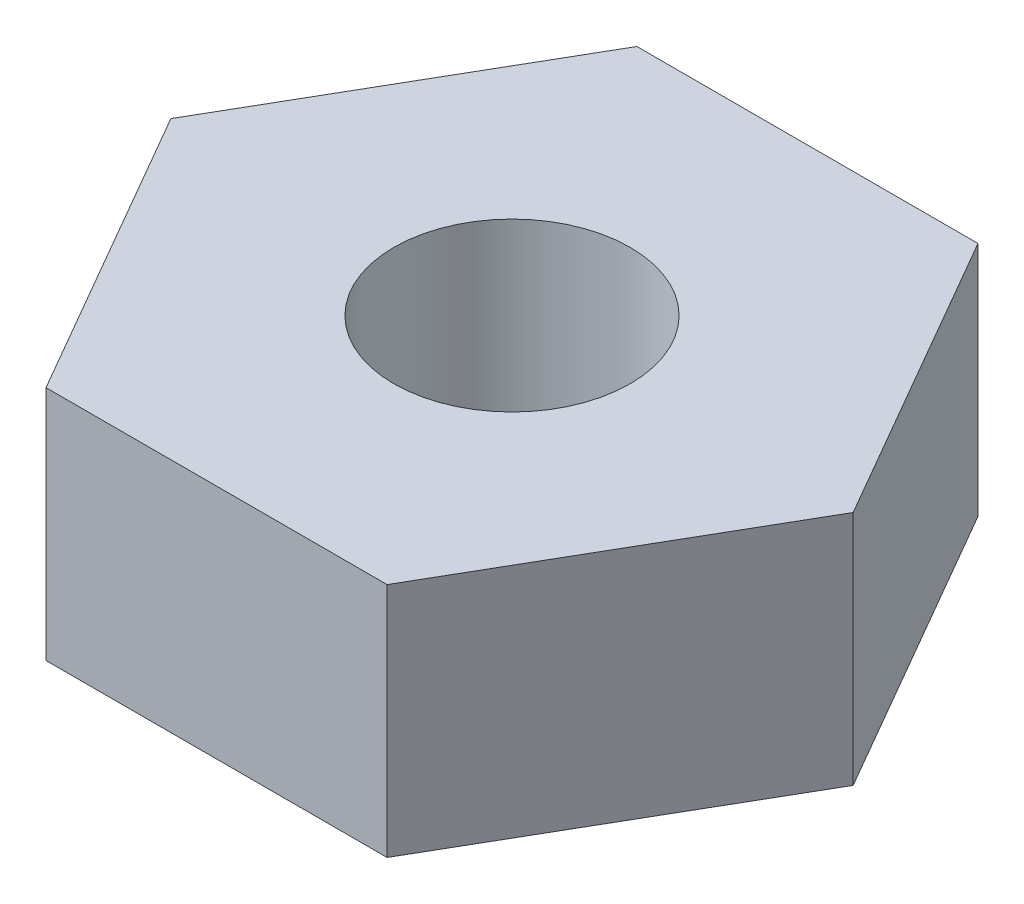
from build123d import *

# Parameters (mm, degrees)
HEX_NUT_PROFILE_R  = 10
HEX_NUT_BODY_DEPTH = 10


with BuildPart() as part:
    # Hex Nut Profile → Hex Nut Body (new, symmetric)
    with BuildSketch(Plane(origin=(0, 0, 0), x_dir=(1, 0, 0), z_dir=(0, 1, 0))):
        Polygon((28.867513459, 0), (14.43375673, 25), (-14.43375673, 25), (-28.867513459, 0), (-14.43375673, -25), (14.43375673, -25), align=None)
        with Locations(Location((0, 0, 0), (0, 0, 270))):
            Circle(HEX_NUT_PROFILE_R, mode=Mode.SUBTRACT)
    extrude(amount=HEX_NUT_BODY_DEPTH, both=True)


solid = part.part
